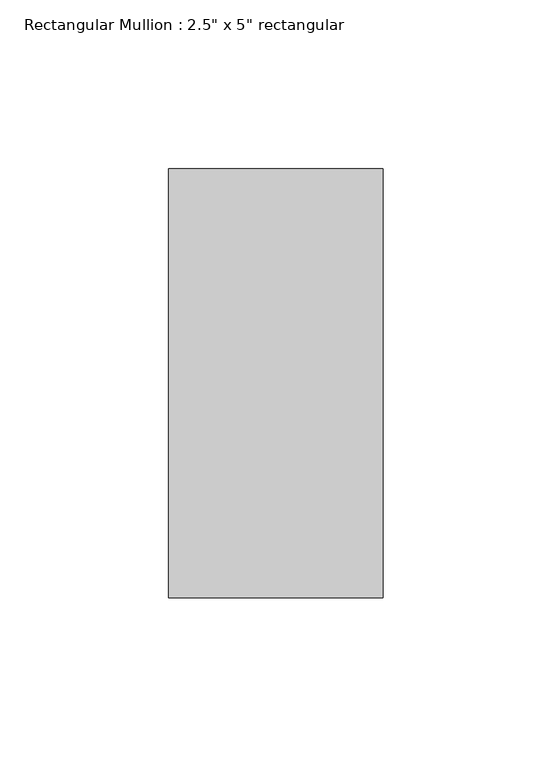
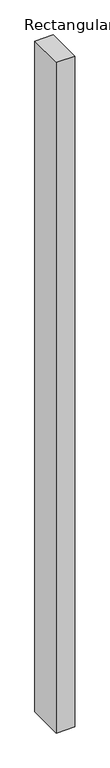
"""IFC4 building model written with IfcOpenShell, lengths in millimetres: member geometry."""

from ifc_helpers import new_model, si_unit, frame, origin, place, context, project, spatial, polyline, outline, extrude, source, transform, mapped, element, save


def member_ccee4eb0(model_context):
    return source(origin(), model_context, "Body", "SweptSolid", [
        extrude(outline(polyline([(0.0, 63.5), (0.0, -63.5), (-63.5, -63.5), (-63.5, 63.5), (0.0, 63.5)])), frame((0.0, 0.0, -2431.9655837), z_axis=(0.0, 0.0, 1.0), x_axis=(1.0, 0.0, 0.0)), (0.0, 0.0, 1.0), 2431.9655837),
    ])


if __name__ == "__main__":
    model = new_model("IFC4")
    model_context = context("Model", 3, world=origin())
    ifc_project = project(units=[si_unit("LENGTHUNIT", "METRE", prefix="MILLI")], contexts=[model_context])
    site = spatial("IfcSite", under=ifc_project)
    building = spatial("IfcBuilding", under=site)
    placement = place(None, origin())
    member_shape = member_ccee4eb0(model_context)
    element("IfcMember", 1, ObjectType="Rectangular Mullion : 2.5\" x 5\" rectangular", at=placement, inside=building, context=model_context, shape_type="MappedRepresentation", body=[
        mapped(member_shape, transform((0.0, 0.0, 0.0), x_axis=(1.0, 0.0, 0.0), y_axis=(0.0, 1.0, 0.0), z_axis=(0.0, 0.0, 1.0))),
    ])
    save(model, "model.ifc")

# Revit data of these elements
# Type "Rectangular Mullion : 2.5\" x 5\" rectangular"
#   built-in parameter 1007304 = 0.416667 (stored number, unit not read)
#   built-in parameter 1007301 = 0.104167 (stored number, unit not read)
#   built-in parameter 1007300 = 0.104167 (stored number, unit not read)
# Element 1 (IfcMember, "Rectangular Mullion : 2.5\" x 5\" rectangular")
#   Materials on its faces: "Aluminum"
# Materials
#   "Aluminum": class "Metal", colour RGB 247 247 247, transparency 0, Description = "Aluminum 6061", Cost = 0
